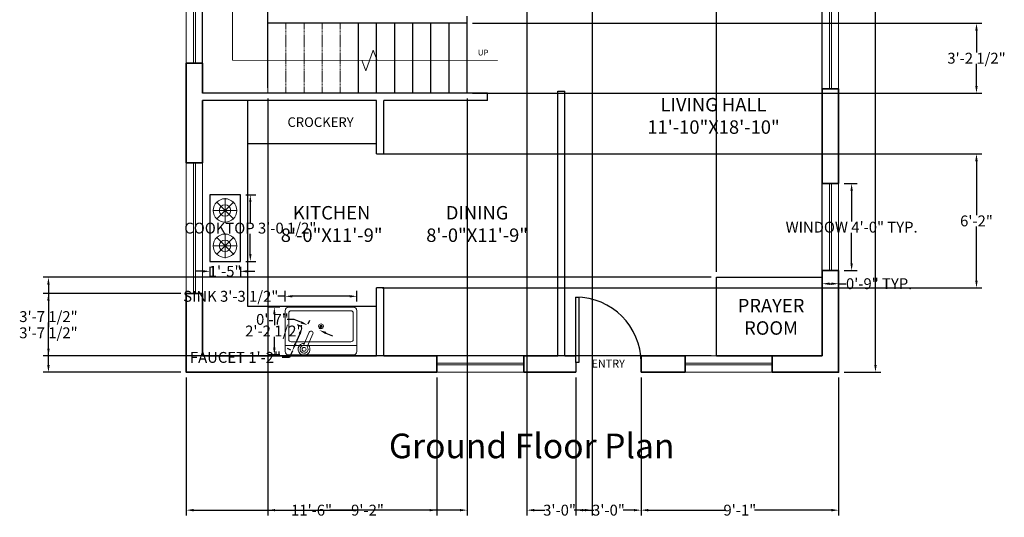
# Model space of a CAD drawing. Units: inches. Extents: x 328 to 872, y 288 to 933.
# Tile 1 of 2: x 328 to 872, y 288 to 562. Entities that reach past the tile are written whole.
import ezdxf

# ---------------------------------------------------------------- set-up
doc = ezdxf.new("R2010")
doc.units = ezdxf.units.IN
doc.header["$MEASUREMENT"] = 0
doc.linetypes.add('DASHED', pattern=[0.75, 0.5, -0.25])
for name, color, linetype, lineweight in [('A-ANNO-DIMS', 2, 'Continuous', 18), ('A-ANNO-SYMB', 7, 'Continuous', 18), ('A-ANNO-TEXT', 7, 'Continuous', 18), ('A-AREA-IDEN', 7, 'Continuous', 18), ('A-FLOR', 7, 'Continuous', 25), ('A-FLOR-CASE', 11, 'Continuous', 25), ('A-FLOR-FIXT', 11, 'Continuous', 18), ('A-FLOR-STRS-OVHD', 30, 'DASHED', 18), ('Doors', 28, 'Continuous', 25), ('Inner Wall', 14, 'Continuous', 30), ('Kitchen Appliances', 11, 'Continuous', 18), ('Outer Wall', 10, 'Continuous', 35), ('Stairs', 30, 'Continuous', 25), ('Windows', 160, 'Continuous', 18)]:
    doc.layers.add(name, color=color, linetype=linetype, lineweight=lineweight)
doc.styles.add('ATTR', font='romans.shx', dxfattribs={"width": 0.8, "height": 1.075})
doc.styles.get("Standard").update_dxf_attribs({"font": 'arial.ttf'})
doc.dimstyles.get("Standard").update_dxf_attribs({"dimtxt": 6, "dimasz": 4, "dimexe": 3, "dimexo": 3, "dimgap": 0.09, "dimtad": 0, "dimtih": 1, "dimtoh": 1, "dimdec": 1, "dimzin": 0, "dimdsep": 46, "dimlunit": 3, "dimtxsty": 'Standard', "dimcen": 0.09, "dimadec": 0, "dimazin": 0, "dimtfac": 1, "dimtdec": 1, "dimtofl": 0, "dimtmove": 0, "dimatfit": 3, "dimfxl": 1, "dimtolj": 1, "dimtzin": 0, "dimarcsym": 0})

# ---------------------------------------------------------------- blocks, each defined once
blk = doc.blocks.new('Gas')
for p, q in [((758.79, 395.85), (755.66, 398.98)), ((758.79, 395.85), (758.79, 400.28)), ((758.79, 395.85), (761.92, 398.98)), ((758.79, 395.85), (754.37, 395.85)), ((758.79, 395.85), (755.66, 392.73)), ((758.79, 395.85), (758.79, 391.43)), ((758.79, 395.85), (761.92, 392.73)), ((758.79, 395.85), (763.22, 395.85)), ((758.79, 383.09), (755.66, 386.22)), ((758.79, 383.09), (758.79, 387.51)), ((758.79, 383.09), (761.92, 386.22)), ((758.79, 383.09), (754.37, 383.09)), ((758.79, 383.09), (755.66, 379.96)), ((758.79, 383.09), (758.79, 378.66)), ((758.79, 383.09), (761.92, 379.96)), ((758.79, 383.09), (763.22, 383.09))]:
    blk.add_line(p, q)
for centre, radius in [((758.79, 395.85), 4.23), ((758.79, 395.85), 2.07), ((758.79, 383.09), 4.23), ((758.79, 383.09), 2.07)]:
    blk.add_circle(centre, radius)
at = {"layer": 'Inner Wall'}
for p, q in [((753.33, 401.47), (753.33, 377.47)), ((764.33, 401.47), (753.33, 401.47)), ((764.33, 377.47), (764.33, 401.47)), ((753.33, 377.47), (764.33, 377.47))]:
    blk.add_line(p, q, dxfattribs=at)
blk = doc.blocks.new("30'' Sink Single PV")
blk.add_line((-15, -3.999996), (15, -3.999996))
for points in [[(-13.5, 0), (13.5, 0)], [(-15, -18.499996), (-15, -1.5)], [(15, -1.5), (15, -18.499996)], [(-13.5, -17.499996), (-13.5, -6.499996)], [(-12.5, -5.499996), (12.5, -5.499996)], [(13.5, -6.499996), (13.5, -17.499996)], [(13.5, -19.999996), (-13.5, -19.999996)], [(12.5, -18.499996), (-12.5, -18.499996)]]:
    blk.add_lwpolyline(points)
for radius in [1, 0.5]:
    blk.add_circle((0, -11.999996), radius)
for centre, radius, start, end in [((-13.5, -1.5), 1.5, 90, 180), ((13.5, -1.5), 1.5, 0, 90), ((-12.5, -6.499996), 1, 90, 180), ((12.5, -6.499996), 1, 0, 90), ((-13.5, -18.499996), 1.5, 180, 270), ((-12.5, -17.499996), 1, 180, 270), ((12.5, -17.499996), 1, 270, 0), ((13.5, -18.499996), 1.5, 270, 0)]:
    blk.add_arc(centre, radius, start, end)
at = {"style": 'ATTR', "width": 0.8, "flags": 9}
blk.add_attdef('ESTCODE', (0, 0), '', height=0.006, dxfattribs=at)
blk = doc.blocks.new('Faucet Top View')
for p, q in [((636.42, 354.98), (636.42, 343.27)), ((639.64, 343.27), (639.64, 354.98))]:
    blk.add_line(p, q)
blk.add_circle((638.03, 357.77), 1.61)
for centre, radius, start, end in [((638.03, 357.77), 4.83, 289.6514, 250.3603), ((638.03, 357.77), 3.22, 300.3431, 239.7554), ((638.03, 343.27), 1.61, 180, 0)]:
    blk.add_arc(centre, radius, start, end)
blk = doc.blocks.new('*U10')
for p, q in [((0, 0), (0, -6)), ((40, 0), (40, -6))]:
    blk.add_line(p, q)
blk.add_lwpolyline([(0, 0), (0, 40), (1.75, 40), (1.75, 0)], close=True)
blk.add_arc((0, 0), 40, 0, 90)
blk = doc.blocks.new('*D12')
at = {"layer": 'A-ANNO-DIMS', "color": 0, "lineweight": -2, "transparency": 16777216}
for p, q in [((783.12, 847.8), (803.48, 847.8)), ((800.48, 843.8), (800.48, 610.95)), ((800.48, 371.8), (800.48, 604.65)), ((783.12, 367.8), (803.48, 367.8))]:
    blk.add_line(p, q, dxfattribs=at)
at = {"layer": 'A-ANNO-DIMS', "color": 0, "transparency": 16777216}
for points in [[(799.82, 843.8), (801.15, 843.8), (800.48, 847.8)], [(799.82, 371.8), (801.15, 371.8), (800.48, 367.8)]]:
    blk.add_solid(points, dxfattribs=at)
at = {"layer": 'Defpoints', "color": 0, "transparency": 16777216}
for p in [(780.12, 847.8), (780.12, 367.8), (800.48, 367.8)]:
    blk.add_point(p, dxfattribs=at)
at = {"layer": 'A-ANNO-DIMS', "color": 0, "transparency": 16777216, "insert": (800.48, 607.8), "char_height": 6, "attachment_point": 5}
blk.add_mtext("\\A1;40'", dxfattribs=at)
blk = doc.blocks.new('WIN-48IN')
for p, q in [((4, 0), (4, 48)), ((5, 48), (5, 0))]:
    blk.add_line(p, q)
blk.add_lwpolyline([(9, 0), (0, 0), (0, 48), (9, 48)], close=True)
blk = doc.blocks.new('WIN-72IN')
for p, q in [((4, 72), (4, 0)), ((5, 72), (5, 0))]:
    blk.add_line(p, q)
blk.add_lwpolyline([(9, 72), (9, 0), (0, 0), (0, 72)], close=True)
blk = doc.blocks.new('*D17')
at = {"layer": 'A-ANNO-DIMS', "color": 0, "lineweight": -2, "transparency": 16777216}
for p, q in [((783.12, 471.84), (790.32, 471.84)), ((787.32, 467.84), (787.32, 451.03)), ((787.32, 427.84), (787.32, 444.64)), ((783.12, 423.84), (790.32, 423.84))]:
    blk.add_line(p, q, dxfattribs=at)
at = {"layer": 'A-ANNO-DIMS', "color": 0, "transparency": 16777216}
for points in [[(786.66, 467.84), (787.99, 467.84), (787.32, 471.84)], [(786.66, 427.84), (787.99, 427.84), (787.32, 423.84)]]:
    blk.add_solid(points, dxfattribs=at)
at = {"layer": 'Defpoints', "color": 0, "transparency": 16777216}
for p in [(780.12, 471.84), (787.32, 471.84), (780.12, 423.84)]:
    blk.add_point(p, dxfattribs=at)
at = {"layer": 'A-ANNO-DIMS', "color": 0, "transparency": 16777216, "insert": (787.32, 447.84), "char_height": 6, "attachment_point": 5}
blk.add_mtext('\\A1;WINDOW 4\'-0" TYP.', dxfattribs=at)
blk = doc.blocks.new('*D18')
at = {"layer": 'A-ANNO-DIMS', "color": 0, "lineweight": -2, "transparency": 16777216}
for p, q in [((771.12, 420.84), (771.12, 413.64)), ((780.12, 420.84), (780.12, 413.64)), ((775.12, 416.64), (776.12, 416.64)), ((780.12, 416.64), (784.12, 416.64))]:
    blk.add_line(p, q, dxfattribs=at)
at = {"layer": 'A-ANNO-DIMS', "color": 0, "transparency": 16777216}
for points in [[(775.12, 417.3), (775.12, 415.97), (771.12, 416.64)], [(776.12, 417.3), (776.12, 415.97), (780.12, 416.64)]]:
    blk.add_solid(points, dxfattribs=at)
at = {"layer": 'Defpoints', "color": 0, "transparency": 16777216}
for p in [(771.12, 423.84), (780.12, 423.84), (780.12, 416.64)]:
    blk.add_point(p, dxfattribs=at)
at = {"layer": 'A-ANNO-DIMS', "color": 0, "transparency": 16777216, "insert": (802.5, 416.64), "char_height": 6, "attachment_point": 5}
blk.add_mtext('\\A1;0\'-9" TYP.', dxfattribs=at)
blk = doc.blocks.new('*D27')
at = {"layer": 'A-ANNO-DIMS', "color": 0, "lineweight": -2, "transparency": 16777216}
for p, q in [((452.94, 465.64), (458.44, 465.64)), ((455.44, 461.64), (455.44, 450.5)), ((455.44, 432.98), (455.44, 444.11)), ((452.94, 428.98), (458.44, 428.98))]:
    blk.add_line(p, q, dxfattribs=at)
at = {"layer": 'A-ANNO-DIMS', "color": 0, "transparency": 16777216}
for points in [[(454.78, 461.64), (456.11, 461.64), (455.44, 465.64)], [(454.78, 432.98), (456.11, 432.98), (455.44, 428.98)]]:
    blk.add_solid(points, dxfattribs=at)
at = {"layer": 'Defpoints', "color": 0, "transparency": 16777216}
for p in [(449.94, 465.64), (455.44, 465.64), (449.94, 428.98)]:
    blk.add_point(p, dxfattribs=at)
at = {"layer": 'A-ANNO-DIMS', "color": 0, "transparency": 16777216, "insert": (455.44, 447.31), "char_height": 6, "attachment_point": 5}
blk.add_mtext('\\A1;COOKTOP 3\'-0 1/2"', dxfattribs=at)
blk = doc.blocks.new('*D28')
at = {"layer": 'A-ANNO-DIMS', "color": 0, "lineweight": -2, "transparency": 16777216}
for p, q in [((433.14, 425.98), (433.14, 420.48)), ((449.94, 425.98), (449.94, 420.48)), ((429.14, 423.48), (425.14, 423.48)), ((453.94, 423.48), (457.94, 423.48))]:
    blk.add_line(p, q, dxfattribs=at)
at = {"layer": 'A-ANNO-DIMS', "color": 0, "transparency": 16777216}
for points in [[(429.14, 424.14), (429.14, 422.81), (433.14, 423.48)], [(453.94, 424.14), (453.94, 422.81), (449.94, 423.48)]]:
    blk.add_solid(points, dxfattribs=at)
at = {"layer": 'Defpoints', "color": 0, "transparency": 16777216}
for p in [(433.14, 428.98), (449.94, 428.98), (449.94, 423.48)]:
    blk.add_point(p, dxfattribs=at)
at = {"layer": 'A-ANNO-DIMS', "color": 0, "transparency": 16777216, "insert": (441.54, 423.48), "char_height": 6, "attachment_point": 5}
blk.add_mtext('\\A1;1\'-5"', dxfattribs=at)
blk = doc.blocks.new('*D29')
at = {"layer": 'A-ANNO-DIMS', "color": 0, "lineweight": -2, "transparency": 16777216}
for p, q in [((474.65, 409.69), (470.65, 409.69)), ((474.65, 406.74), (474.65, 412.69)), ((510.28, 409.69), (478.65, 409.69)), ((514.28, 406.74), (514.28, 412.69))]:
    blk.add_line(p, q, dxfattribs=at)
at = {"layer": 'A-ANNO-DIMS', "color": 0, "transparency": 16777216}
for points in [[(478.65, 410.36), (478.65, 409.02), (474.65, 409.69)], [(510.28, 410.36), (510.28, 409.02), (514.28, 409.69)]]:
    blk.add_solid(points, dxfattribs=at)
at = {"layer": 'Defpoints', "color": 0, "transparency": 16777216}
for p in [(474.65, 409.69), (474.65, 403.74), (514.28, 403.74)]:
    blk.add_point(p, dxfattribs=at)
at = {"layer": 'A-ANNO-DIMS', "color": 0, "transparency": 16777216, "insert": (444.66, 409.69), "char_height": 6, "attachment_point": 5}
blk.add_mtext('\\A1;SINK 3\'-3 1/2"', dxfattribs=at)
blk = doc.blocks.new('*D30')
at = {"layer": 'A-ANNO-DIMS', "color": 0, "lineweight": -2, "transparency": 16777216}
for p, q in [((471.65, 403.74), (465.7, 403.74)), ((468.7, 399.74), (468.7, 393.72)), ((468.7, 381.31), (468.7, 387.34)), ((471.65, 377.31), (465.7, 377.31))]:
    blk.add_line(p, q, dxfattribs=at)
at = {"layer": 'A-ANNO-DIMS', "color": 0, "transparency": 16777216}
for points in [[(468.04, 399.74), (469.37, 399.74), (468.7, 403.74)], [(468.04, 381.31), (469.37, 381.31), (468.7, 377.31)]]:
    blk.add_solid(points, dxfattribs=at)
at = {"layer": 'Defpoints', "color": 0, "transparency": 16777216}
for p in [(474.65, 403.74), (468.7, 377.31), (474.65, 377.31)]:
    blk.add_point(p, dxfattribs=at)
at = {"layer": 'A-ANNO-DIMS', "color": 0, "transparency": 16777216, "insert": (468.7, 390.53), "char_height": 6, "attachment_point": 5}
blk.add_mtext('\\A1;2\'-2 1/2"', dxfattribs=at)
blk = doc.blocks.new('*D31')
at = {"layer": 'A-ANNO-DIMS', "color": 0, "lineweight": -2, "transparency": 16777216}
for p, q in [((483.46, 393.02), (481.51, 393.86)), ((482.68, 389), (480.24, 383.33)), ((477.85, 380), (475.9, 380.84)), ((477.07, 375.98), (473.07, 375.98)), ((478.66, 379.65), (477.07, 375.98))]:
    blk.add_line(p, q, dxfattribs=at)
at = {"layer": 'A-ANNO-DIMS', "color": 0, "transparency": 16777216}
for points in [[(482.07, 389.27), (483.29, 388.74), (484.26, 392.68)], [(479.63, 383.59), (480.85, 383.06), (478.66, 379.65)]]:
    blk.add_solid(points, dxfattribs=at)
at = {"layer": 'Defpoints', "color": 0, "transparency": 16777216}
for p in [(486.22, 391.83), (478.66, 379.65), (480.61, 378.81)]:
    blk.add_point(p, dxfattribs=at)
at = {"layer": 'A-ANNO-DIMS', "color": 0, "transparency": 16777216, "insert": (447.25, 375.98), "char_height": 6, "attachment_point": 5}
blk.add_mtext('\\A1;FAUCET 1\'-2"', dxfattribs=at)
blk = doc.blocks.new('*D32')
at = {"layer": 'A-ANNO-DIMS', "color": 0, "lineweight": -2, "transparency": 16777216}
for p, q in [((479.71, 396.95), (475.71, 396.95)), ((483.38, 395.37), (479.71, 396.95)), ((487.4, 394.59), (488.24, 396.54)), ((493.82, 391.82), (494.66, 393.78)), ((497.15, 389.44), (500.83, 387.86))]:
    blk.add_line(p, q, dxfattribs=at)
at = {"layer": 'A-ANNO-DIMS', "color": 0, "transparency": 16777216}
for points in [[(483.65, 395.98), (483.12, 394.76), (487.06, 393.79)], [(497.42, 390.05), (496.89, 388.83), (493.48, 391.02)]]:
    blk.add_solid(points, dxfattribs=at)
at = {"layer": 'Defpoints', "color": 0, "transparency": 16777216}
for p in [(486.22, 391.83), (487.06, 393.79), (492.64, 389.07)]:
    blk.add_point(p, dxfattribs=at)
at = {"layer": 'A-ANNO-DIMS', "color": 0, "transparency": 16777216, "insert": (467.65, 396.95), "char_height": 6, "attachment_point": 5}
blk.add_mtext('\\A1;0\'-7"', dxfattribs=at)
blk = doc.blocks.new('*D33')
at = {"layer": 'A-ANNO-DIMS', "color": 0, "lineweight": -2, "transparency": 16777216}
for p, q in [((635.12, 364.8), (635.12, 288.7)), ((671.12, 364.8), (671.12, 288.7)), ((639.12, 291.7), (645.06, 291.7)), ((667.12, 291.7), (661.19, 291.7))]:
    blk.add_line(p, q, dxfattribs=at)
at = {"layer": 'A-ANNO-DIMS', "color": 0, "transparency": 16777216}
for points in [[(639.12, 292.36), (639.12, 291.03), (635.12, 291.7)], [(667.12, 292.36), (667.12, 291.03), (671.12, 291.7)]]:
    blk.add_solid(points, dxfattribs=at)
at = {"layer": 'Defpoints', "color": 0, "transparency": 16777216}
for p in [(635.12, 367.8), (671.12, 367.8), (671.12, 291.7)]:
    blk.add_point(p, dxfattribs=at)
at = {"layer": 'A-ANNO-DIMS', "color": 0, "transparency": 16777216, "insert": (653.12, 291.7), "char_height": 6, "attachment_point": 5}
blk.add_mtext('\\A1;3\'-0"', dxfattribs=at)
blk = doc.blocks.new('*D34')
at = {"layer": 'A-ANNO-DIMS', "color": 0, "lineweight": -2, "transparency": 16777216}
for p, q in [((671.12, 364.8), (671.12, 288.7)), ((780.12, 364.8), (780.12, 288.7)), ((675.12, 291.7), (717.56, 291.7)), ((776.12, 291.7), (733.69, 291.7))]:
    blk.add_line(p, q, dxfattribs=at)
at = {"layer": 'A-ANNO-DIMS', "color": 0, "transparency": 16777216}
for points in [[(675.12, 292.36), (675.12, 291.03), (671.12, 291.7)], [(776.12, 292.36), (776.12, 291.03), (780.12, 291.7)]]:
    blk.add_solid(points, dxfattribs=at)
at = {"layer": 'Defpoints', "color": 0, "transparency": 16777216}
for p in [(671.12, 367.8), (780.12, 367.8), (780.12, 291.7)]:
    blk.add_point(p, dxfattribs=at)
at = {"layer": 'A-ANNO-DIMS', "color": 0, "transparency": 16777216, "insert": (725.62, 291.7), "char_height": 6, "attachment_point": 5}
blk.add_mtext('\\A1;9\'-1"', dxfattribs=at)
blk = doc.blocks.new('*D35')
at = {"layer": 'A-ANNO-DIMS', "color": 0, "lineweight": -2, "transparency": 16777216}
for p, q in [((712.72, 423.18), (712.72, 926.91)), ((716.72, 923.91), (724.42, 923.91)), ((767.12, 923.91), (759.43, 923.91)), ((771.12, 423.18), (771.12, 926.91))]:
    blk.add_line(p, q, dxfattribs=at)
at = {"layer": 'A-ANNO-DIMS', "color": 0, "transparency": 16777216}
for points in [[(716.72, 924.57), (716.72, 923.24), (712.72, 923.91)], [(767.12, 924.57), (767.12, 923.24), (771.12, 923.91)]]:
    blk.add_solid(points, dxfattribs=at)
at = {"layer": 'Defpoints', "color": 0, "transparency": 16777216}
for p in [(771.12, 923.91), (712.72, 420.18), (771.12, 420.18)]:
    blk.add_point(p, dxfattribs=at)
at = {"layer": 'A-ANNO-DIMS', "color": 0, "transparency": 16777216, "insert": (741.92, 923.91), "char_height": 6, "attachment_point": 5}
blk.add_mtext('\\A1;4\'-10 1/2"', dxfattribs=at)
blk = doc.blocks.new('*D36')
at = {"layer": 'A-ANNO-DIMS', "color": 0, "lineweight": -2, "transparency": 16777216}
for p, q in [((709.72, 420.18), (341.02, 420.18)), ((344.02, 416.18), (344.02, 401.68)), ((344.02, 380.8), (344.02, 395.3)), ((709.72, 376.8), (341.02, 376.8))]:
    blk.add_line(p, q, dxfattribs=at)
at = {"layer": 'A-ANNO-DIMS', "color": 0, "transparency": 16777216}
for points in [[(343.35, 416.18), (344.68, 416.18), (344.02, 420.18)], [(343.35, 380.8), (344.68, 380.8), (344.02, 376.8)]]:
    blk.add_solid(points, dxfattribs=at)
at = {"layer": 'Defpoints', "color": 0, "transparency": 16777216}
for p in [(344.02, 420.18), (712.72, 420.18), (712.72, 376.8)]:
    blk.add_point(p, dxfattribs=at)
at = {"layer": 'A-ANNO-DIMS', "color": 0, "transparency": 16777216, "insert": (344.02, 398.49), "char_height": 6, "attachment_point": 5}
blk.add_mtext('\\A1;3\'-7 1/2"', dxfattribs=at)
blk = doc.blocks.new('*D37')
at = {"layer": 'A-ANNO-DIMS', "color": 0, "lineweight": -2, "transparency": 16777216}
for p, q in [((608.12, 667.8), (608.12, 288.7)), ((644.12, 667.8), (644.12, 288.7)), ((612.12, 291.7), (618.06, 291.7)), ((640.12, 291.7), (634.19, 291.7))]:
    blk.add_line(p, q, dxfattribs=at)
at = {"layer": 'A-ANNO-DIMS', "color": 0, "transparency": 16777216}
for points in [[(612.12, 292.36), (612.12, 291.03), (608.12, 291.7)], [(640.12, 292.36), (640.12, 291.03), (644.12, 291.7)]]:
    blk.add_solid(points, dxfattribs=at)
at = {"layer": 'Defpoints', "color": 0, "transparency": 16777216}
for p in [(608.12, 670.8), (644.12, 670.8), (644.12, 291.7)]:
    blk.add_point(p, dxfattribs=at)
at = {"layer": 'A-ANNO-DIMS', "color": 0, "transparency": 16777216, "insert": (626.12, 291.7), "char_height": 6, "attachment_point": 5}
blk.add_mtext('\\A1;3\'-0"', dxfattribs=at)
blk = doc.blocks.new('*D40')
at = {"layer": 'A-ANNO-DIMS', "color": 0, "lineweight": -2, "transparency": 16777216}
for p, q in [((420.12, 364.8), (420.12, 288.7)), ((558.36, 364.8), (558.36, 288.7)), ((424.12, 291.7), (479.13, 291.7)), ((554.36, 291.7), (499.36, 291.7))]:
    blk.add_line(p, q, dxfattribs=at)
at = {"layer": 'A-ANNO-DIMS', "color": 0, "transparency": 16777216}
for points in [[(424.12, 292.36), (424.12, 291.03), (420.12, 291.7)], [(554.36, 292.36), (554.36, 291.03), (558.36, 291.7)]]:
    blk.add_solid(points, dxfattribs=at)
at = {"layer": 'Defpoints', "color": 0, "transparency": 16777216}
for p in [(420.12, 367.8), (558.36, 367.8), (558.36, 291.7)]:
    blk.add_point(p, dxfattribs=at)
at = {"layer": 'A-ANNO-DIMS', "color": 0, "transparency": 16777216, "insert": (489.24, 291.7), "char_height": 6, "attachment_point": 5}
blk.add_mtext('\\A1;11\'-6"', dxfattribs=at)
blk = doc.blocks.new('*D41')
at = {"layer": 'A-ANNO-DIMS', "color": 0, "lineweight": -2, "transparency": 16777216}
for p, q in [((417.12, 411.28), (341.02, 411.28)), ((344.02, 407.28), (344.02, 392.73)), ((344.02, 371.8), (344.02, 386.34)), ((417.12, 367.8), (341.02, 367.8))]:
    blk.add_line(p, q, dxfattribs=at)
at = {"layer": 'A-ANNO-DIMS', "color": 0, "transparency": 16777216}
for points in [[(343.35, 407.28), (344.68, 407.28), (344.02, 411.28)], [(343.35, 371.8), (344.68, 371.8), (344.02, 367.8)]]:
    blk.add_solid(points, dxfattribs=at)
at = {"layer": 'Defpoints', "color": 0, "transparency": 16777216}
for p in [(344.02, 411.28), (420.12, 411.28), (420.12, 367.8)]:
    blk.add_point(p, dxfattribs=at)
at = {"layer": 'A-ANNO-DIMS', "color": 0, "transparency": 16777216, "insert": (344.02, 389.54), "char_height": 6, "attachment_point": 5}
blk.add_mtext('\\A1;3\'-7 1/2"', dxfattribs=at)
blk = doc.blocks.new('*D42')
at = {"layer": 'A-ANNO-DIMS', "color": 0, "lineweight": -2, "transparency": 16777216}
for p, q in [((528.12, 488.24), (859.23, 488.24)), ((856.23, 484.24), (856.23, 454.43)), ((856.23, 418.31), (856.23, 448.12)), ((528.12, 414.31), (859.23, 414.31))]:
    blk.add_line(p, q, dxfattribs=at)
at = {"layer": 'A-ANNO-DIMS', "color": 0, "transparency": 16777216}
for points in [[(855.56, 484.24), (856.89, 484.24), (856.23, 488.24)], [(855.56, 418.31), (856.89, 418.31), (856.23, 414.31)]]:
    blk.add_solid(points, dxfattribs=at)
at = {"layer": 'Defpoints', "color": 0, "transparency": 16777216}
for p in [(525.12, 488.24), (856.23, 488.24), (525.12, 414.31)]:
    blk.add_point(p, dxfattribs=at)
at = {"layer": 'A-ANNO-DIMS', "color": 0, "transparency": 16777216, "insert": (856.23, 451.28), "char_height": 6, "attachment_point": 5}
blk.add_mtext('\\A1;6\'-2"', dxfattribs=at)
blk = doc.blocks.new('*D43')
at = {"layer": 'A-ANNO-DIMS', "color": 0, "lineweight": -2, "transparency": 16777216}
for p, q in [((429.12, 524.8), (429.12, 926.91)), ((433.12, 923.91), (439.06, 923.91)), ((461.12, 923.91), (455.19, 923.91)), ((465.12, 524.8), (465.12, 926.91))]:
    blk.add_line(p, q, dxfattribs=at)
at = {"layer": 'A-ANNO-DIMS', "color": 0, "transparency": 16777216}
for points in [[(433.12, 924.57), (433.12, 923.24), (429.12, 923.91)], [(461.12, 924.57), (461.12, 923.24), (465.12, 923.91)]]:
    blk.add_solid(points, dxfattribs=at)
at = {"layer": 'Defpoints', "color": 0, "transparency": 16777216}
for p in [(465.12, 923.91), (429.12, 521.8), (465.12, 521.8)]:
    blk.add_point(p, dxfattribs=at)
at = {"layer": 'A-ANNO-DIMS', "color": 0, "transparency": 16777216, "insert": (447.12, 923.91), "char_height": 6, "attachment_point": 5}
blk.add_mtext('\\A1;3\'-0"', dxfattribs=at)
blk = doc.blocks.new('*D44')
at = {"layer": 'A-ANNO-DIMS', "color": 0, "lineweight": -2, "transparency": 16777216}
for p, q in [((465.12, 518.8), (465.12, 288.7)), ((575.12, 518.8), (575.12, 288.7)), ((469.12, 291.7), (512.06, 291.7)), ((571.12, 291.7), (528.19, 291.7))]:
    blk.add_line(p, q, dxfattribs=at)
at = {"layer": 'A-ANNO-DIMS', "color": 0, "transparency": 16777216}
for points in [[(469.12, 292.36), (469.12, 291.03), (465.12, 291.7)], [(571.12, 292.36), (571.12, 291.03), (575.12, 291.7)]]:
    blk.add_solid(points, dxfattribs=at)
at = {"layer": 'Defpoints', "color": 0, "transparency": 16777216}
for p in [(465.12, 521.8), (575.12, 521.8), (575.12, 291.7)]:
    blk.add_point(p, dxfattribs=at)
at = {"layer": 'A-ANNO-DIMS', "color": 0, "transparency": 16777216, "insert": (520.12, 291.7), "char_height": 6, "attachment_point": 5}
blk.add_mtext('\\A1;9\'-2"', dxfattribs=at)
blk = doc.blocks.new('*D45')
at = {"layer": 'A-ANNO-DIMS', "color": 0, "lineweight": -2, "transparency": 16777216}
for p, q in [((578.12, 560.3), (859.23, 560.3)), ((856.23, 556.3), (856.23, 544.25)), ((856.23, 525.8), (856.23, 537.86)), ((578.12, 521.8), (859.23, 521.8))]:
    blk.add_line(p, q, dxfattribs=at)
at = {"layer": 'A-ANNO-DIMS', "color": 0, "transparency": 16777216}
for points in [[(855.56, 556.3), (856.89, 556.3), (856.23, 560.3)], [(855.56, 525.8), (856.89, 525.8), (856.23, 521.8)]]:
    blk.add_solid(points, dxfattribs=at)
at = {"layer": 'Defpoints', "color": 0, "transparency": 16777216}
for p in [(575.12, 560.3), (856.23, 560.3), (575.12, 521.8)]:
    blk.add_point(p, dxfattribs=at)
at = {"layer": 'A-ANNO-DIMS', "color": 0, "transparency": 16777216, "insert": (856.23, 541.05), "char_height": 6, "attachment_point": 5}
blk.add_mtext('\\A1;3\'-2 1/2"', dxfattribs=at)

msp = doc.modelspace()

# ---------------------------------------------------------------- linework, layer by layer
at = {"layer": 'A-ANNO-SYMB'}
for p, q in [((445.67, 540.02), (445.67, 582.8)), ((591.87, 539.75), (445.67, 540.02))]:
    msp.add_line(p, q, dxfattribs=at)
msp.add_lwpolyline([(517.07, 539.89), (519.13, 534.18), (523.31, 545.58), (525.37, 539.87)], dxfattribs=at)
at = {"layer": 'A-FLOR'}
msp.add_lwpolyline([(712.72, 420.18), (771.12, 420.18), (771.12, 376.8), (712.72, 376.8)], close=True, dxfattribs=at)
at = {"layer": 'A-FLOR-CASE'}
for p, q in [((453.84, 517.8), (453.84, 404.3)), ((453.84, 493.98), (525.12, 493.98)), ((453.84, 404.3), (525.12, 404.3))]:
    msp.add_line(p, q, dxfattribs=at)
at = {"layer": 'A-FLOR-STRS-OVHD'}
for p, q in [((465.12, 521.8), (465.12, 602.8)), ((475.12, 521.8), (475.12, 560.3)), ((485.12, 521.8), (485.12, 560.3)), ((495.12, 521.8), (495.12, 560.3)), ((505.12, 521.8), (505.12, 560.3))]:
    msp.add_line(p, q, dxfattribs=at)
at = {"layer": 'Inner Wall'}
for p, q in [((586.34, 521.8), (429.12, 521.8)), ((586.34, 517.8), (586.34, 521.8)), ((625.12, 376.8), (625.12, 522.8)), ((625.12, 522.8), (629.12, 522.8)), ((629.12, 376.8), (629.12, 522.8)), ((525.12, 517.8), (429.12, 517.8)), ((525.12, 488.24), (525.12, 517.8)), ((529.12, 488.24), (529.12, 517.8)), ((586.34, 517.8), (529.12, 517.8)), ((525.12, 488.24), (529.12, 488.24)), ((525.12, 376.8), (525.12, 414.31)), ((529.12, 414.31), (525.12, 414.31)), ((529.12, 376.8), (529.12, 414.31))]:
    msp.add_line(p, q, dxfattribs=at)
at = {"layer": 'Outer Wall'}
for p, q in [((429.12, 538.36), (420.12, 538.36)), ((429.12, 521.8), (429.12, 538.36)), ((771.12, 524.17), (780.12, 524.17)), ((771.12, 524.17), (771.12, 471.84)), ((429.12, 483.28), (429.12, 517.8)), ((429.12, 483.28), (420.12, 483.28)), ((771.12, 471.84), (780.12, 471.84)), ((771.12, 423.84), (780.12, 423.84)), ((771.12, 423.84), (771.12, 376.8)), ((429.12, 411.28), (420.12, 411.28)), ((429.12, 376.8), (429.12, 411.28)), ((525.12, 376.8), (429.12, 376.8)), ((558.36, 376.8), (529.12, 376.8)), ((558.36, 367.8), (558.36, 376.8)), ((606.36, 367.8), (606.36, 376.8)), ((625.12, 376.8), (606.36, 376.8)), ((635.12, 376.8), (629.12, 376.8)), ((671.12, 367.8), (671.12, 376.8)), ((695.5, 376.8), (671.12, 376.8)), ((695.5, 367.8), (695.5, 376.8)), ((771.12, 376.8), (712.72, 376.8)), ((743.5, 367.8), (743.5, 376.8))]:
    msp.add_line(p, q, dxfattribs=at)
for points in [[(420.12, 483.28), (420.12, 538.36)], [(780.12, 524.17), (780.12, 471.84)], [(780.12, 423.84), (780.12, 367.8), (743.5, 367.8)], [(558.36, 367.8), (420.12, 367.8), (420.12, 411.28)], [(635.12, 367.8), (606.36, 367.8)], [(695.5, 367.8), (671.12, 367.8)]]:
    msp.add_lwpolyline(points, dxfattribs=at)
at = {"layer": 'Stairs'}
for p, q in [((575.12, 560.3), (465.12, 560.3)), ((515.12, 521.8), (515.12, 560.3)), ((525.12, 521.8), (525.12, 560.3)), ((535.12, 521.8), (535.12, 560.3)), ((545.12, 521.8), (545.12, 560.3)), ((555.12, 521.8), (555.12, 560.3)), ((565.12, 521.8), (565.12, 560.3)), ((575.12, 521.8), (575.12, 564.3))]:
    msp.add_line(p, q, dxfattribs=at)

# ---------------------------------------------------------------- block references
at = {"layer": 'A-FLOR-FIXT'}
for name, p, xscale, yscale, zscale, rotation in [("30'' Sink Single PV", (494.46, 377.32), 1.321146747817903, 1.321146747817903, 1.321146747817903, 180), ('Faucet Top View', (977.71, 432.05), 0.6770973782848909, 0.6770973782848909, 0.6770973782848909, 156.7008130032402)]:
    msp.add_blockref(name, p, dxfattribs=dict(at, xscale=xscale, yscale=yscale, zscale=zscale, rotation=rotation))
at = {"layer": 'Doors', "xscale": 0.900000000000003, "yscale": 0.900000000000003, "zscale": 0.900000000000003}
msp.add_blockref('*U10', (635.12, 373.2), dxfattribs=at)
at = {"layer": 'Kitchen Appliances', "xscale": 1.527598045333809, "yscale": 1.527598045333809, "zscale": 1.527598045333809}
msp.add_blockref('Gas', (-717.65, -147.65), dxfattribs=at)
at = {"layer": 'Windows'}
for name, p in [('WIN-48IN', (420.12, 538.36)), ('WIN-48IN', (771.12, 524.17)), ('WIN-72IN', (420.12, 411.27)), ('WIN-48IN', (771.12, 423.84))]:
    msp.add_blockref(name, p, dxfattribs=at)
for p, rotation in [((606.36, 367.8), 90.00000000000011), ((743.5, 367.8), 90.00000000000031)]:
    msp.add_blockref('WIN-48IN', p, dxfattribs=dict(at, rotation=rotation))

# ---------------------------------------------------------------- texts
at = {"layer": 'A-ANNO-TEXT', "attachment_point": 1}
for s, width, gutter_width, insert, char_height in [('\\pxqc;{UP}', 143.6128, 15.71, (512.13, 545.71), 3.141), ('\\pxqc;CROCKERY', 1074.0317, 26.51, (-42.81, 508.43), 5.3021), ('\\pxqc;{\\fCascadia Code|b1|i0|c0|p49;ENTRY}', 791.5735, 21.99, (257.16, 374.77), 4.3976), ('\\pxqc;{\\fArial|b1|i0|c0|p34;Ground Floor Plan}', 2755.0414, 68, (-766.79, 333.94), 13.6006)]:
    msp.add_mtext_dynamic_manual_height_columns(s, width=width, gutter_width=gutter_width, heights=[0], dxfattribs=dict(at, insert=insert, char_height=char_height))
at = {"layer": 'A-AREA-IDEN', "char_height": 7.4254, "attachment_point": 1}
for s, insert in [('\\pxqc;LIVING HALL\\P11\'-10"X18\'-10"', (-40.99, 519.15)), ('\\pxqc;KITCHEN\\P8\'-0"X11\'-9"', (-251.75, 459.49)), ('\\pxqc;DINING\\P8\'-0"X11\'-9"', (-171.46, 459.49)), ('\\pxqc;PRAYER\\PROOM', (-9.23, 408.29))]:
    msp.add_mtext_dynamic_manual_height_columns(s, width=1504.1481, gutter_width=37.13, heights=[0], dxfattribs=dict(at, insert=insert))

# ---------------------------------------------------------------- dimensions: what is measured, and where the dimension line sits
at = {"layer": 'A-ANNO-DIMS'}
for base, p1, p2, picture, middle in [((771.12, 923.91), (712.72, 420.18), (771.12, 420.18), '*D35', (741.92, 923.91)), ((465.12, 923.91), (429.12, 521.8), (465.12, 521.8), '*D43', (447.12, 923.91)), ((644.12, 291.7), (608.12, 670.8), (644.12, 670.8), '*D37', (626.12, 291.7)), ((575.12, 291.7), (465.12, 521.8), (575.12, 521.8), '*D44', (520.12, 291.7)), ((449.94, 423.48), (433.14, 428.98), (449.94, 428.98), '*D28', (441.54, 423.48)), ((558.36, 291.7), (420.12, 367.8), (558.36, 367.8), '*D40', (489.24, 291.7)), ((671.12, 291.7), (635.12, 367.8), (671.12, 367.8), '*D33', (653.12, 291.7)), ((780.12, 291.7), (671.12, 367.8), (780.12, 367.8), '*D34', (725.62, 291.7))]:
    dim = msp.add_linear_dim(base=base, p1=p1, p2=p2, dimstyle='Standard', override={"dimdec": 1, "dimlfac": 1, "dimrnd": 0, "dimzin": 1, "dimdsep": 46, "dimlunit": 4, "dimfrac": 2}, dxfattribs=at)
    dim.commit()
    dim.dimension.update_dxf_attribs({"geometry": picture, "text_midpoint": middle})
for base, p1, p2, angle, override, picture, middle in [((800.48, 367.8), (780.12, 847.8), (780.12, 367.8), 90, {"dimclrd": 0, "dimclre": 0, "dimclrt": 0}, '*D12', (800.48, 607.8)), ((856.23, 560.3), (575.12, 521.8), (575.12, 560.3), 90, {"dimdec": 1, "dimlfac": 1, "dimrnd": 0, "dimzin": 1, "dimdsep": 46, "dimlunit": 4, "dimfrac": 2}, '*D45', (856.23, 541.05)), ((856.23, 488.24), (525.12, 414.31), (525.12, 488.24), 90, {"dimdec": 1, "dimlfac": 1, "dimrnd": 0, "dimzin": 1, "dimdsep": 46, "dimlunit": 4, "dimfrac": 2}, '*D42', (856.23, 451.28)), ((344.02, 420.18), (712.72, 376.8), (712.72, 420.18), 90, {"dimdec": 1, "dimlfac": 1, "dimrnd": 0, "dimzin": 1, "dimdsep": 46, "dimlunit": 4, "dimfrac": 2}, '*D36', (344.02, 398.49)), ((344.02, 411.28), (420.12, 367.8), (420.12, 411.28), 90, {"dimdec": 1, "dimlfac": 1, "dimrnd": 0, "dimzin": 1, "dimdsep": 46, "dimlunit": 4, "dimfrac": 2}, '*D41', (344.02, 389.54)), ((468.7, 377.31), (474.65, 403.74), (474.65, 377.31), 270, {"dimdec": 1, "dimlfac": 1, "dimrnd": 0, "dimzin": 1, "dimdsep": 46, "dimlunit": 4, "dimfrac": 2}, '*D30', (468.7, 390.53)), ((487.06, 393.79), (492.64, 389.07), (486.22, 391.83), 156.7008, {"dimdec": 1, "dimlfac": 1, "dimrnd": 0, "dimzin": 1, "dimdsep": 46, "dimlunit": 4, "dimfrac": 2}, '*D32', (467.65, 396.95))]:
    dim = msp.add_linear_dim(base=base, p1=p1, p2=p2, angle=angle, dimstyle='Standard', override=override, dxfattribs=at)
    dim.commit()
    dim.dimension.update_dxf_attribs({"geometry": picture, "text_midpoint": middle})
for base, p1, p2, angle, text, picture, middle in [((787.32, 471.84), (780.12, 423.84), (780.12, 471.84), 90, 'WINDOW <> TYP.', '*D17', (787.32, 447.84)), ((455.44, 465.64), (449.94, 428.98), (449.94, 465.64), 90, 'COOKTOP <>', '*D27', (455.44, 447.31)), ((474.65, 409.69), (514.28, 403.74), (474.65, 403.74), 180, 'SINK <>', '*D29', (444.66, 409.69)), ((478.66, 379.65), (486.22, 391.83), (480.61, 378.81), 246.7008, 'FAUCET <>', '*D31', (447.25, 375.98))]:
    dim = msp.add_linear_dim(base=base, p1=p1, p2=p2, angle=angle, text=text, dimstyle='Standard', override={"dimdec": 1, "dimlfac": 1, "dimrnd": 0, "dimzin": 1, "dimdsep": 46, "dimlunit": 4, "dimfrac": 2}, dxfattribs=at)
    dim.commit()
    dim.dimension.update_dxf_attribs({"geometry": picture, "text_midpoint": middle})
dim = msp.add_linear_dim(base=(780.12, 416.64), p1=(771.12, 423.84), p2=(780.12, 423.84), text='<> TYP.', dimstyle='Standard', override={"dimdec": 1, "dimlfac": 1, "dimrnd": 0, "dimzin": 1, "dimdsep": 46, "dimlunit": 4, "dimfrac": 2}, dxfattribs=at)
dim.commit()
dim.dimension.update_dxf_attribs({"geometry": '*D18', "text_midpoint": (802.5, 416.64)})

doc.saveas('drawing.dxf')
